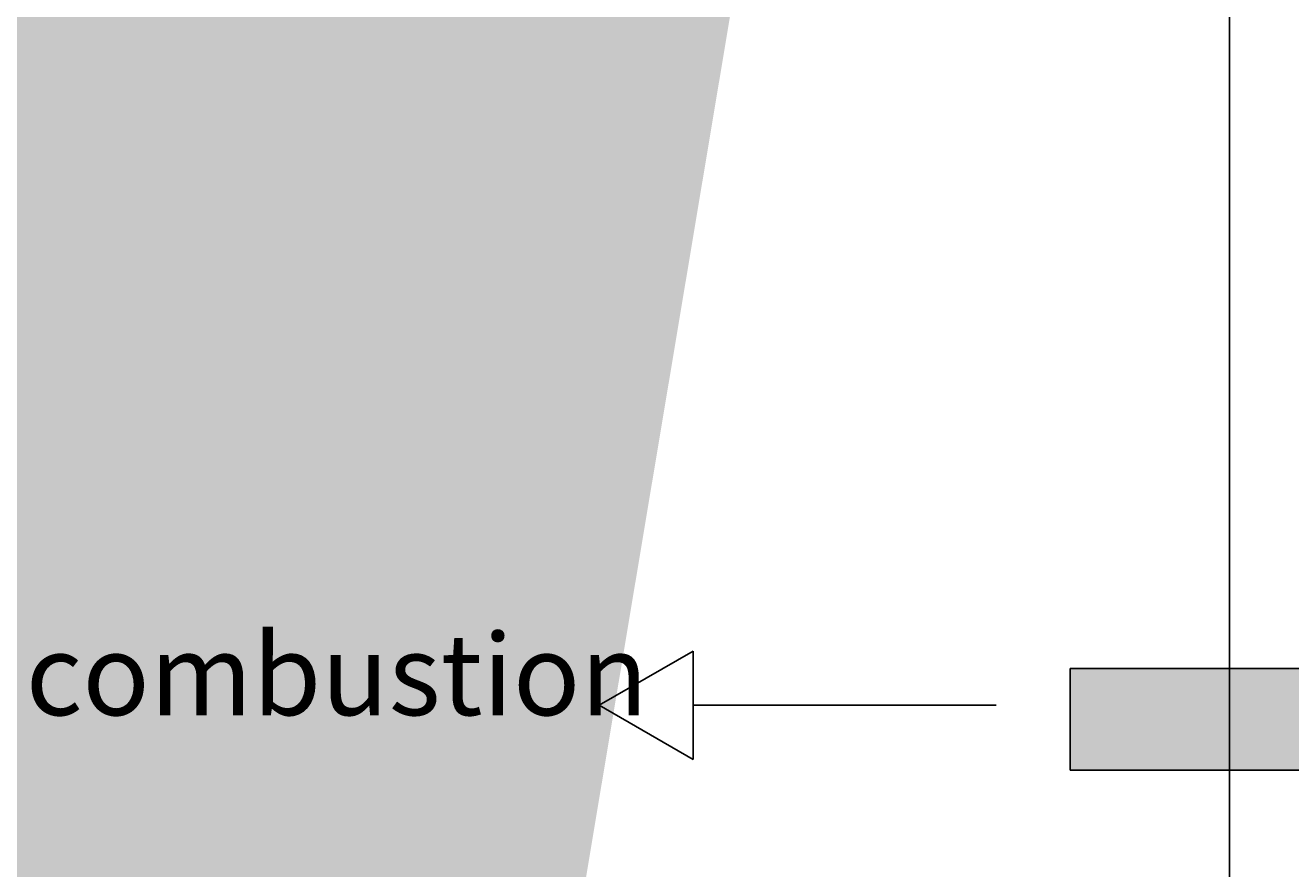
# Model space of a CAD drawing. Units: millimetres. Extents: x -22994 to 29398, y -19990 to 20176.
# Tile 25 of 135: x 37 to 99, y 138 to 180. Entities that reach past the tile are written whole.
import ezdxf

# ---------------------------------------------------------------- set-up
doc = ezdxf.new("R2010")
doc.units = ezdxf.units.MM
doc.header["$MEASUREMENT"] = 0
for name, color, linetype, lineweight in [('M-ANNO-SYMB', 7, 'Continuous', 25), ('M-ANNO-TEXT', 7, 'Continuous', 25), ('M-DIMS', 2, 'Continuous', 18), ('M-EQPM', 7, 'Continuous', 25), ('M-EQPM-PATT', 7, 'Continuous', 18)]:
    doc.layers.add(name, color=color, linetype=linetype, lineweight=lineweight)
doc.styles.get("Standard").update_dxf_attribs({"font": 'arial.ttf'})
doc.dimstyles.get("Standard").update_dxf_attribs({"dimtxt": 0.18, "dimasz": 10000, "dimexe": 0.18, "dimexo": 0.0625, "dimgap": 0.09, "dimtad": 0, "dimtih": 1, "dimtoh": 1, "dimdec": 0, "dimzin": 0, "dimdsep": 46, "dimtxsty": 'Standard', "dimcen": 0.09, "dimadec": 0, "dimazin": 0, "dimtfac": 1, "dimtdec": 0, "dimtofl": 0, "dimtmove": 0, "dimatfit": 3, "dimfxl": 1, "dimtolj": 1, "dimtzin": 0, "dimlwd": 30, "dimarcsym": 0})

# ---------------------------------------------------------------- blocks, each defined once
blk = doc.blocks.new('ARROW-FLOW')
for p, q in [((4.609, 5.322), (0, 2.661)), ((4.609, 5.322), (4.609, 0)), ((4.609, 0), (0, 2.661))]:
    blk.add_line(p, q)
blk = doc.blocks.new('*D2')
at = {"layer": 'Defpoints', "color": 0, "transparency": 16777216}
for p in [(6.677, 10.271), (290.852, 10.271), (290.852, -5.079)]:
    blk.add_point(p, dxfattribs=at)
at = {"layer": 'M-DIMS', "color": 0, "lineweight": -2, "transparency": 16777216}
for p, q in [((6.677, 10.209), (6.677, -5.259)), ((290.852, 10.209), (290.852, -5.259))]:
    blk.add_line(p, q, dxfattribs=at)
at = {"layer": 'M-DIMS', "color": 0, "lineweight": 30, "transparency": 16777216}
for p, q in [((-9993.323, -5.079), (-19993.323, -5.079)), ((10290.852, -5.079), (20290.852, -5.079))]:
    blk.add_line(p, q, dxfattribs=at)
at = {"layer": 'M-DIMS', "color": 0, "transparency": 16777216}
for points in [[(-9993.323, 1661.588), (-9993.323, -1671.745), (6.677, -5.079)], [(10290.852, 1661.588), (10290.852, -1671.745), (290.852, -5.079)]]:
    blk.add_solid(points, dxfattribs=at)
at = {"layer": 'M-DIMS', "color": 0, "transparency": 16777216, "insert": (148.765, -5.079), "char_height": 0.18, "attachment_point": 5}
blk.add_mtext('\\A1;284.2', dxfattribs=at)
blk = doc.blocks.new('*D3')
at = {"layer": 'Defpoints', "color": 0, "transparency": 16777216}
for p in [(110.265, 204.165), (110.265, 176.366), (95.833, 127.967)]:
    blk.add_point(p, dxfattribs=at)
at = {"layer": 'M-DIMS', "color": 0, "lineweight": 30, "transparency": 16777216}
for p, q in [((-9904.167, 204.165), (-19904.167, 204.165)), ((10110.265, 204.165), (20110.265, 204.165))]:
    blk.add_line(p, q, dxfattribs=at)
at = {"layer": 'M-DIMS', "color": 0, "lineweight": -2, "transparency": 16777216}
for p, q in [((95.833, 128.03), (95.833, 204.345)), ((110.265, 176.429), (110.265, 204.345))]:
    blk.add_line(p, q, dxfattribs=at)
at = {"layer": 'M-DIMS', "color": 0, "transparency": 16777216}
for points in [[(-9904.167, 1870.832), (-9904.167, -1462.501), (95.833, 204.165)], [(10110.265, 1870.832), (10110.265, -1462.501), (110.265, 204.165)]]:
    blk.add_solid(points, dxfattribs=at)
at = {"layer": 'M-DIMS', "color": 0, "transparency": 16777216, "insert": (103.049, 204.165), "char_height": 0.18, "attachment_point": 5}
blk.add_mtext('\\A1;14.432', dxfattribs=at)
blk = doc.blocks.new('*D4')
at = {"layer": 'Defpoints', "color": 0, "transparency": 16777216}
for p in [(116.265, 204.165), (110.265, 176.366), (116.265, 176.366)]:
    blk.add_point(p, dxfattribs=at)
at = {"layer": 'M-DIMS', "color": 0, "lineweight": 30, "transparency": 16777216}
for p, q in [((-9889.735, 204.165), (-19889.735, 204.165)), ((10116.265, 204.165), (20116.265, 204.165))]:
    blk.add_line(p, q, dxfattribs=at)
at = {"layer": 'M-DIMS', "color": 0, "lineweight": -2, "transparency": 16777216}
for p, q in [((110.265, 176.429), (110.265, 204.345)), ((116.265, 176.429), (116.265, 204.345))]:
    blk.add_line(p, q, dxfattribs=at)
at = {"layer": 'M-DIMS', "color": 0, "transparency": 16777216}
for points in [[(-9889.735, 1870.832), (-9889.735, -1462.501), (110.265, 204.165)], [(10116.265, 1870.832), (10116.265, -1462.501), (116.265, 204.165)]]:
    blk.add_solid(points, dxfattribs=at)
at = {"layer": 'M-DIMS', "color": 0, "transparency": 16777216, "insert": (113.265, 204.165), "char_height": 0.18, "attachment_point": 5}
blk.add_mtext('\\A1;6', dxfattribs=at)
blk = doc.blocks.new('*D5')
at = {"layer": 'Defpoints', "color": 0, "transparency": 16777216}
for p in [(181.265, 204.165), (116.265, 176.366), (181.265, 176.366)]:
    blk.add_point(p, dxfattribs=at)
at = {"layer": 'M-DIMS', "color": 0, "lineweight": 30, "transparency": 16777216}
for p, q in [((-9883.735, 204.165), (-19883.735, 204.165)), ((10181.265, 204.165), (20181.265, 204.165))]:
    blk.add_line(p, q, dxfattribs=at)
at = {"layer": 'M-DIMS', "color": 0, "lineweight": -2, "transparency": 16777216}
for p, q in [((116.265, 176.429), (116.265, 204.345)), ((181.265, 176.429), (181.265, 204.345))]:
    blk.add_line(p, q, dxfattribs=at)
at = {"layer": 'M-DIMS', "color": 0, "transparency": 16777216}
for points in [[(-9883.735, 1870.832), (-9883.735, -1462.501), (116.265, 204.165)], [(10181.265, 1870.832), (10181.265, -1462.501), (181.265, 204.165)]]:
    blk.add_solid(points, dxfattribs=at)
at = {"layer": 'M-DIMS', "color": 0, "transparency": 16777216, "insert": (148.765, 204.165), "char_height": 0.18, "attachment_point": 5}
blk.add_mtext('\\A1;65', dxfattribs=at)
blk = doc.blocks.new('*D6')
at = {"layer": 'Defpoints', "color": 0, "transparency": 16777216}
for p in [(187.265, 204.165), (181.265, 176.366), (187.265, 176.366)]:
    blk.add_point(p, dxfattribs=at)
at = {"layer": 'M-DIMS', "color": 0, "lineweight": 30, "transparency": 16777216}
for p, q in [((-9818.735, 204.165), (-19818.735, 204.165)), ((10187.265, 204.165), (20187.265, 204.165))]:
    blk.add_line(p, q, dxfattribs=at)
at = {"layer": 'M-DIMS', "color": 0, "lineweight": -2, "transparency": 16777216}
for p, q in [((181.265, 176.429), (181.265, 204.345)), ((187.265, 176.429), (187.265, 204.345))]:
    blk.add_line(p, q, dxfattribs=at)
at = {"layer": 'M-DIMS', "color": 0, "transparency": 16777216}
for points in [[(-9818.735, 1870.832), (-9818.735, -1462.501), (181.265, 204.165)], [(10187.265, 1870.832), (10187.265, -1462.501), (187.265, 204.165)]]:
    blk.add_solid(points, dxfattribs=at)
at = {"layer": 'M-DIMS', "color": 0, "transparency": 16777216, "insert": (184.265, 204.165), "char_height": 0.18, "attachment_point": 5}
blk.add_mtext('\\A1;6', dxfattribs=at)
blk = doc.blocks.new('*D7')
at = {"layer": 'Defpoints', "color": 0, "transparency": 16777216}
for p in [(201.697, 204.165), (187.265, 176.366), (201.697, 127.967)]:
    blk.add_point(p, dxfattribs=at)
at = {"layer": 'M-DIMS', "color": 0, "lineweight": 30, "transparency": 16777216}
for p, q in [((-9812.735, 204.165), (-19812.735, 204.165)), ((10201.697, 204.165), (20201.697, 204.165))]:
    blk.add_line(p, q, dxfattribs=at)
at = {"layer": 'M-DIMS', "color": 0, "lineweight": -2, "transparency": 16777216}
for p, q in [((187.265, 176.429), (187.265, 204.345)), ((201.697, 128.03), (201.697, 204.345))]:
    blk.add_line(p, q, dxfattribs=at)
at = {"layer": 'M-DIMS', "color": 0, "transparency": 16777216}
for points in [[(-9812.735, 1870.832), (-9812.735, -1462.501), (187.265, 204.165)], [(10201.697, 1870.832), (10201.697, -1462.501), (201.697, 204.165)]]:
    blk.add_solid(points, dxfattribs=at)
at = {"layer": 'M-DIMS', "color": 0, "transparency": 16777216, "insert": (194.481, 204.165), "char_height": 0.18, "attachment_point": 5}
blk.add_mtext('\\A1;14.432', dxfattribs=at)
blk = doc.blocks.new('*D8')
at = {"layer": 'Defpoints', "color": 0, "transparency": 16777216}
for p in [(227.648, 204.165), (227.648, 146.73), (201.697, 127.967)]:
    blk.add_point(p, dxfattribs=at)
at = {"layer": 'M-DIMS', "color": 0, "lineweight": 30, "transparency": 16777216}
for p, q in [((-9798.303, 204.165), (-19798.303, 204.165)), ((10227.648, 204.165), (20227.648, 204.165))]:
    blk.add_line(p, q, dxfattribs=at)
at = {"layer": 'M-DIMS', "color": 0, "lineweight": -2, "transparency": 16777216}
for p, q in [((201.697, 128.03), (201.697, 204.345)), ((227.648, 146.792), (227.648, 204.345))]:
    blk.add_line(p, q, dxfattribs=at)
at = {"layer": 'M-DIMS', "color": 0, "transparency": 16777216}
for points in [[(-9798.303, 1870.832), (-9798.303, -1462.501), (201.697, 204.165)], [(10227.648, 1870.832), (10227.648, -1462.501), (227.648, 204.165)]]:
    blk.add_solid(points, dxfattribs=at)
at = {"layer": 'M-DIMS', "color": 0, "transparency": 16777216, "insert": (214.673, 204.165), "char_height": 0.18, "attachment_point": 5}
blk.add_mtext('\\A1;25.95', dxfattribs=at)
blk = doc.blocks.new('*D9')
at = {"layer": 'Defpoints', "color": 0, "transparency": 16777216}
for p in [(187.265, 176.366), (306.202, 176.366), (290.852, 10.271)]:
    blk.add_point(p, dxfattribs=at)
at = {"layer": 'M-DIMS', "color": 0, "lineweight": 30, "transparency": 16777216}
for p, q in [((306.202, 10176.366), (306.202, 20176.366)), ((306.202, -9989.729), (306.202, -19989.729))]:
    blk.add_line(p, q, dxfattribs=at)
at = {"layer": 'M-DIMS', "color": 0, "lineweight": -2, "transparency": 16777216}
for p, q in [((187.327, 176.366), (306.382, 176.366)), ((290.915, 10.271), (306.382, 10.271))]:
    blk.add_line(p, q, dxfattribs=at)
at = {"layer": 'M-DIMS', "color": 0, "transparency": 16777216}
for points in [[(-1360.465, 10176.366), (1972.869, 10176.366), (306.202, 176.366)], [(-1360.465, -9989.729), (1972.869, -9989.729), (306.202, 10.271)]]:
    blk.add_solid(points, dxfattribs=at)
at = {"layer": 'M-DIMS', "color": 0, "transparency": 16777216, "insert": (306.202, 93.319), "char_height": 0.18, "attachment_point": 5}
blk.add_mtext('\\A1;166.1', dxfattribs=at)
blk = doc.blocks.new('*D10')
at = {"layer": 'Defpoints', "color": 0, "transparency": 16777216}
for p in [(125.65, 136.071), (133.346, 136.071), (133.346, -5.079)]:
    blk.add_point(p, dxfattribs=at)
at = {"layer": 'M-DIMS', "color": 0, "lineweight": -2, "transparency": 16777216}
for p, q in [((125.65, 136.009), (125.65, -5.259)), ((133.346, 136.009), (133.346, -5.259))]:
    blk.add_line(p, q, dxfattribs=at)
at = {"layer": 'M-DIMS', "color": 0, "lineweight": 30, "transparency": 16777216}
for p, q in [((-9874.35, -5.079), (-19874.35, -5.079)), ((10133.346, -5.079), (20133.346, -5.079))]:
    blk.add_line(p, q, dxfattribs=at)
at = {"layer": 'M-DIMS', "color": 0, "transparency": 16777216}
for points in [[(-9874.35, 1661.588), (-9874.35, -1671.745), (125.65, -5.079)], [(10133.346, 1661.588), (10133.346, -1671.745), (133.346, -5.079)]]:
    blk.add_solid(points, dxfattribs=at)
at = {"layer": 'M-DIMS', "color": 0, "transparency": 16777216, "insert": (129.498, -5.079), "char_height": 0.18, "attachment_point": 5}
blk.add_mtext('\\A1;7.696', dxfattribs=at)
blk = doc.blocks.new('*D11')
at = {"layer": 'Defpoints', "color": 0, "transparency": 16777216}
for p in [(133.346, 136.071), (135.65, 136.071), (135.65, -5.079)]:
    blk.add_point(p, dxfattribs=at)
at = {"layer": 'M-DIMS', "color": 0, "lineweight": -2, "transparency": 16777216}
for p, q in [((133.346, 136.009), (133.346, -5.259)), ((135.65, 136.009), (135.65, -5.259))]:
    blk.add_line(p, q, dxfattribs=at)
at = {"layer": 'M-DIMS', "color": 0, "lineweight": 30, "transparency": 16777216}
for p, q in [((-9866.654, -5.079), (-19866.654, -5.079)), ((10135.65, -5.079), (20135.65, -5.079))]:
    blk.add_line(p, q, dxfattribs=at)
at = {"layer": 'M-DIMS', "color": 0, "transparency": 16777216}
for points in [[(-9866.654, 1661.588), (-9866.654, -1671.745), (133.346, -5.079)], [(10135.65, 1661.588), (10135.65, -1671.745), (135.65, -5.079)]]:
    blk.add_solid(points, dxfattribs=at)
at = {"layer": 'M-DIMS', "color": 0, "transparency": 16777216, "insert": (134.498, -5.079), "char_height": 0.18, "attachment_point": 5}
blk.add_mtext('\\A1;2.304', dxfattribs=at)
blk = doc.blocks.new('*D12')
at = {"layer": 'Defpoints', "color": 0, "transparency": 16777216}
for p in [(135.65, 136.071), (145.65, 136.071), (145.65, -5.079)]:
    blk.add_point(p, dxfattribs=at)
at = {"layer": 'M-DIMS', "color": 0, "lineweight": -2, "transparency": 16777216}
for p, q in [((135.65, 136.009), (135.65, -5.259)), ((145.65, 136.009), (145.65, -5.259))]:
    blk.add_line(p, q, dxfattribs=at)
at = {"layer": 'M-DIMS', "color": 0, "lineweight": 30, "transparency": 16777216}
for p, q in [((-9864.35, -5.079), (-19864.35, -5.079)), ((10145.65, -5.079), (20145.65, -5.079))]:
    blk.add_line(p, q, dxfattribs=at)
at = {"layer": 'M-DIMS', "color": 0, "transparency": 16777216}
for points in [[(-9864.35, 1661.588), (-9864.35, -1671.745), (135.65, -5.079)], [(10145.65, 1661.588), (10145.65, -1671.745), (145.65, -5.079)]]:
    blk.add_solid(points, dxfattribs=at)
at = {"layer": 'M-DIMS', "color": 0, "transparency": 16777216, "insert": (140.65, -5.079), "char_height": 0.18, "attachment_point": 5}
blk.add_mtext('\\A1;10', dxfattribs=at)
blk = doc.blocks.new('*D13')
at = {"layer": 'Defpoints', "color": 0, "transparency": 16777216}
for p in [(145.65, 136.071), (155.65, 136.071), (155.65, -5.079)]:
    blk.add_point(p, dxfattribs=at)
at = {"layer": 'M-DIMS', "color": 0, "lineweight": -2, "transparency": 16777216}
for p, q in [((145.65, 136.009), (145.65, -5.259)), ((155.65, 136.009), (155.65, -5.259))]:
    blk.add_line(p, q, dxfattribs=at)
at = {"layer": 'M-DIMS', "color": 0, "lineweight": 30, "transparency": 16777216}
for p, q in [((-9854.35, -5.079), (-19854.35, -5.079)), ((10155.65, -5.079), (20155.65, -5.079))]:
    blk.add_line(p, q, dxfattribs=at)
at = {"layer": 'M-DIMS', "color": 0, "transparency": 16777216}
for points in [[(-9854.35, 1661.588), (-9854.35, -1671.745), (145.65, -5.079)], [(10155.65, 1661.588), (10155.65, -1671.745), (155.65, -5.079)]]:
    blk.add_solid(points, dxfattribs=at)
at = {"layer": 'M-DIMS', "color": 0, "transparency": 16777216, "insert": (150.65, -5.079), "char_height": 0.18, "attachment_point": 5}
blk.add_mtext('\\A1;10', dxfattribs=at)
blk = doc.blocks.new('*D14')
at = {"layer": 'Defpoints', "color": 0, "transparency": 16777216}
for p in [(155.65, 136.071), (165.65, 136.071), (165.65, -5.079)]:
    blk.add_point(p, dxfattribs=at)
at = {"layer": 'M-DIMS', "color": 0, "lineweight": -2, "transparency": 16777216}
for p, q in [((155.65, 136.009), (155.65, -5.259)), ((165.65, 136.009), (165.65, -5.259))]:
    blk.add_line(p, q, dxfattribs=at)
at = {"layer": 'M-DIMS', "color": 0, "lineweight": 30, "transparency": 16777216}
for p, q in [((-9844.35, -5.079), (-19844.35, -5.079)), ((10165.65, -5.079), (20165.65, -5.079))]:
    blk.add_line(p, q, dxfattribs=at)
at = {"layer": 'M-DIMS', "color": 0, "transparency": 16777216}
for points in [[(-9844.35, 1661.588), (-9844.35, -1671.745), (155.65, -5.079)], [(10165.65, 1661.588), (10165.65, -1671.745), (165.65, -5.079)]]:
    blk.add_solid(points, dxfattribs=at)
at = {"layer": 'M-DIMS', "color": 0, "transparency": 16777216, "insert": (160.65, -5.079), "char_height": 0.18, "attachment_point": 5}
blk.add_mtext('\\A1;10', dxfattribs=at)
blk = doc.blocks.new('*D15')
at = {"layer": 'Defpoints', "color": 0, "transparency": 16777216}
for p in [(173.346, 154.788), (173.346, 136.071), (306.202, 136.071)]:
    blk.add_point(p, dxfattribs=at)
at = {"layer": 'M-DIMS', "color": 0, "lineweight": 30, "transparency": 16777216}
for p, q in [((306.202, 10154.788), (306.202, 20154.788)), ((306.202, -9863.929), (306.202, -19863.929))]:
    blk.add_line(p, q, dxfattribs=at)
at = {"layer": 'M-DIMS', "color": 0, "lineweight": -2, "transparency": 16777216}
for p, q in [((173.408, 154.788), (306.382, 154.788)), ((173.408, 136.071), (306.382, 136.071))]:
    blk.add_line(p, q, dxfattribs=at)
at = {"layer": 'M-DIMS', "color": 0, "transparency": 16777216}
for points in [[(-1360.465, 10154.788), (1972.869, 10154.788), (306.202, 154.788)], [(-1360.465, -9863.929), (1972.869, -9863.929), (306.202, 136.071)]]:
    blk.add_solid(points, dxfattribs=at)
at = {"layer": 'M-DIMS', "color": 0, "transparency": 16777216, "insert": (306.202, 145.43), "char_height": 0.18, "attachment_point": 5}
blk.add_mtext('\\A1;18.717', dxfattribs=at)
blk = doc.blocks.new('*D16')
at = {"layer": 'Defpoints', "color": 0, "transparency": 16777216}
for p in [(120.17, 204.165), (110.466, 48.035), (120.17, 48.035)]:
    blk.add_point(p, dxfattribs=at)
at = {"layer": 'M-DIMS', "color": 0, "lineweight": 30, "transparency": 16777216}
for p, q in [((-9889.534, 204.165), (-19889.534, 204.165)), ((10120.17, 204.165), (20120.17, 204.165))]:
    blk.add_line(p, q, dxfattribs=at)
at = {"layer": 'M-DIMS', "color": 0, "lineweight": -2, "transparency": 16777216}
for p, q in [((110.466, 48.097), (110.466, 204.345)), ((120.17, 48.097), (120.17, 204.345))]:
    blk.add_line(p, q, dxfattribs=at)
at = {"layer": 'M-DIMS', "color": 0, "transparency": 16777216}
for points in [[(-9889.534, 1870.832), (-9889.534, -1462.501), (110.466, 204.165)], [(10120.17, 1870.832), (10120.17, -1462.501), (120.17, 204.165)]]:
    blk.add_solid(points, dxfattribs=at)
at = {"layer": 'M-DIMS', "color": 0, "transparency": 16777216, "insert": (115.318, 204.165), "char_height": 0.18, "attachment_point": 5}
blk.add_mtext('\\A1;9.704', dxfattribs=at)
blk = doc.blocks.new('*D17')
at = {"layer": 'Defpoints', "color": 0, "transparency": 16777216}
for p in [(126.17, 204.165), (120.17, 48.035), (126.17, 48.035)]:
    blk.add_point(p, dxfattribs=at)
at = {"layer": 'M-DIMS', "color": 0, "lineweight": 30, "transparency": 16777216}
for p, q in [((-9879.83, 204.165), (-19879.83, 204.165)), ((10126.17, 204.165), (20126.17, 204.165))]:
    blk.add_line(p, q, dxfattribs=at)
at = {"layer": 'M-DIMS', "color": 0, "lineweight": -2, "transparency": 16777216}
for p, q in [((120.17, 48.097), (120.17, 204.345)), ((126.17, 48.097), (126.17, 204.345))]:
    blk.add_line(p, q, dxfattribs=at)
at = {"layer": 'M-DIMS', "color": 0, "transparency": 16777216}
for points in [[(-9879.83, 1870.832), (-9879.83, -1462.501), (120.17, 204.165)], [(10126.17, 1870.832), (10126.17, -1462.501), (126.17, 204.165)]]:
    blk.add_solid(points, dxfattribs=at)
at = {"layer": 'M-DIMS', "color": 0, "transparency": 16777216, "insert": (123.17, 204.165), "char_height": 0.18, "attachment_point": 5}
blk.add_mtext('\\A1;6', dxfattribs=at)
blk = doc.blocks.new('*D18')
at = {"layer": 'Defpoints', "color": 0, "transparency": 16777216}
for p in [(132.17, 204.165), (126.17, 48.035), (132.17, 48.035)]:
    blk.add_point(p, dxfattribs=at)
at = {"layer": 'M-DIMS', "color": 0, "lineweight": 30, "transparency": 16777216}
for p, q in [((-9873.83, 204.165), (-19873.83, 204.165)), ((10132.17, 204.165), (20132.17, 204.165))]:
    blk.add_line(p, q, dxfattribs=at)
at = {"layer": 'M-DIMS', "color": 0, "lineweight": -2, "transparency": 16777216}
for p, q in [((126.17, 48.097), (126.17, 204.345)), ((132.17, 48.097), (132.17, 204.345))]:
    blk.add_line(p, q, dxfattribs=at)
at = {"layer": 'M-DIMS', "color": 0, "transparency": 16777216}
for points in [[(-9873.83, 1870.832), (-9873.83, -1462.501), (126.17, 204.165)], [(10132.17, 1870.832), (10132.17, -1462.501), (132.17, 204.165)]]:
    blk.add_solid(points, dxfattribs=at)
at = {"layer": 'M-DIMS', "color": 0, "transparency": 16777216, "insert": (129.17, 204.165), "char_height": 0.18, "attachment_point": 5}
blk.add_mtext('\\A1;6', dxfattribs=at)
blk = doc.blocks.new('*D19')
at = {"layer": 'Defpoints', "color": 0, "transparency": 16777216}
for p in [(138.17, 204.165), (132.17, 48.035), (138.17, 48.035)]:
    blk.add_point(p, dxfattribs=at)
at = {"layer": 'M-DIMS', "color": 0, "lineweight": 30, "transparency": 16777216}
for p, q in [((-9867.83, 204.165), (-19867.83, 204.165)), ((10138.17, 204.165), (20138.17, 204.165))]:
    blk.add_line(p, q, dxfattribs=at)
at = {"layer": 'M-DIMS', "color": 0, "lineweight": -2, "transparency": 16777216}
for p, q in [((132.17, 48.097), (132.17, 204.345)), ((138.17, 48.097), (138.17, 204.345))]:
    blk.add_line(p, q, dxfattribs=at)
at = {"layer": 'M-DIMS', "color": 0, "transparency": 16777216}
for points in [[(-9867.83, 1870.832), (-9867.83, -1462.501), (132.17, 204.165)], [(10138.17, 1870.832), (10138.17, -1462.501), (138.17, 204.165)]]:
    blk.add_solid(points, dxfattribs=at)
at = {"layer": 'M-DIMS', "color": 0, "transparency": 16777216, "insert": (135.17, 204.165), "char_height": 0.18, "attachment_point": 5}
blk.add_mtext('\\A1;6', dxfattribs=at)
blk = doc.blocks.new('*D20')
at = {"layer": 'Defpoints', "color": 0, "transparency": 16777216}
for p in [(144.17, 204.165), (138.17, 48.035), (144.17, 48.035)]:
    blk.add_point(p, dxfattribs=at)
at = {"layer": 'M-DIMS', "color": 0, "lineweight": 30, "transparency": 16777216}
for p, q in [((-9861.83, 204.165), (-19861.83, 204.165)), ((10144.17, 204.165), (20144.17, 204.165))]:
    blk.add_line(p, q, dxfattribs=at)
at = {"layer": 'M-DIMS', "color": 0, "lineweight": -2, "transparency": 16777216}
for p, q in [((138.17, 48.097), (138.17, 204.345)), ((144.17, 48.097), (144.17, 204.345))]:
    blk.add_line(p, q, dxfattribs=at)
at = {"layer": 'M-DIMS', "color": 0, "transparency": 16777216}
for points in [[(-9861.83, 1870.832), (-9861.83, -1462.501), (138.17, 204.165)], [(10144.17, 1870.832), (10144.17, -1462.501), (144.17, 204.165)]]:
    blk.add_solid(points, dxfattribs=at)
at = {"layer": 'M-DIMS', "color": 0, "transparency": 16777216, "insert": (141.17, 204.165), "char_height": 0.18, "attachment_point": 5}
blk.add_mtext('\\A1;6', dxfattribs=at)
blk = doc.blocks.new('*D21')
at = {"layer": 'Defpoints', "color": 0, "transparency": 16777216}
for p in [(149.116, 204.165), (144.17, 48.035), (149.116, 48.035)]:
    blk.add_point(p, dxfattribs=at)
at = {"layer": 'M-DIMS', "color": 0, "lineweight": 30, "transparency": 16777216}
for p, q in [((-9855.83, 204.165), (-19855.83, 204.165)), ((10149.116, 204.165), (20149.116, 204.165))]:
    blk.add_line(p, q, dxfattribs=at)
at = {"layer": 'M-DIMS', "color": 0, "lineweight": -2, "transparency": 16777216}
for p, q in [((144.17, 48.097), (144.17, 204.345)), ((149.116, 48.097), (149.116, 204.345))]:
    blk.add_line(p, q, dxfattribs=at)
at = {"layer": 'M-DIMS', "color": 0, "transparency": 16777216}
for points in [[(-9855.83, 1870.832), (-9855.83, -1462.501), (144.17, 204.165)], [(10149.116, 1870.832), (10149.116, -1462.501), (149.116, 204.165)]]:
    blk.add_solid(points, dxfattribs=at)
at = {"layer": 'M-DIMS', "color": 0, "transparency": 16777216, "insert": (146.643, 204.165), "char_height": 0.18, "attachment_point": 5}
blk.add_mtext('\\A1;4.945', dxfattribs=at)
blk = doc.blocks.new('*D22')
at = {"layer": 'Defpoints', "color": 0, "transparency": 16777216}
for p in [(149.116, 30.99), (155.116, 30.99), (155.116, -5.079)]:
    blk.add_point(p, dxfattribs=at)
at = {"layer": 'M-DIMS', "color": 0, "lineweight": -2, "transparency": 16777216}
for p, q in [((149.116, 30.927), (149.116, -5.259)), ((155.116, 30.927), (155.116, -5.259))]:
    blk.add_line(p, q, dxfattribs=at)
at = {"layer": 'M-DIMS', "color": 0, "lineweight": 30, "transparency": 16777216}
for p, q in [((-9850.884, -5.079), (-19850.884, -5.079)), ((10155.116, -5.079), (20155.116, -5.079))]:
    blk.add_line(p, q, dxfattribs=at)
at = {"layer": 'M-DIMS', "color": 0, "transparency": 16777216}
for points in [[(-9850.884, 1661.588), (-9850.884, -1671.745), (149.116, -5.079)], [(10155.116, 1661.588), (10155.116, -1671.745), (155.116, -5.079)]]:
    blk.add_solid(points, dxfattribs=at)
at = {"layer": 'M-DIMS', "color": 0, "transparency": 16777216, "insert": (152.116, -5.079), "char_height": 0.18, "attachment_point": 5}
blk.add_mtext('\\A1;6', dxfattribs=at)
blk = doc.blocks.new('*D23')
at = {"layer": 'Defpoints', "color": 0, "transparency": 16777216}
for p in [(155.116, 30.99), (161.116, 30.99), (161.116, -5.079)]:
    blk.add_point(p, dxfattribs=at)
at = {"layer": 'M-DIMS', "color": 0, "lineweight": -2, "transparency": 16777216}
for p, q in [((155.116, 30.927), (155.116, -5.259)), ((161.116, 30.927), (161.116, -5.259))]:
    blk.add_line(p, q, dxfattribs=at)
at = {"layer": 'M-DIMS', "color": 0, "lineweight": 30, "transparency": 16777216}
for p, q in [((-9844.884, -5.079), (-19844.884, -5.079)), ((10161.116, -5.079), (20161.116, -5.079))]:
    blk.add_line(p, q, dxfattribs=at)
at = {"layer": 'M-DIMS', "color": 0, "transparency": 16777216}
for points in [[(-9844.884, 1661.588), (-9844.884, -1671.745), (155.116, -5.079)], [(10161.116, 1661.588), (10161.116, -1671.745), (161.116, -5.079)]]:
    blk.add_solid(points, dxfattribs=at)
at = {"layer": 'M-DIMS', "color": 0, "transparency": 16777216, "insert": (158.116, -5.079), "char_height": 0.18, "attachment_point": 5}
blk.add_mtext('\\A1;6', dxfattribs=at)
blk = doc.blocks.new('*D24')
at = {"layer": 'Defpoints', "color": 0, "transparency": 16777216}
for p in [(161.116, 30.99), (166.439, 30.99), (166.439, -5.079)]:
    blk.add_point(p, dxfattribs=at)
at = {"layer": 'M-DIMS', "color": 0, "lineweight": -2, "transparency": 16777216}
for p, q in [((161.116, 30.927), (161.116, -5.259)), ((166.439, 30.927), (166.439, -5.259))]:
    blk.add_line(p, q, dxfattribs=at)
at = {"layer": 'M-DIMS', "color": 0, "lineweight": 30, "transparency": 16777216}
for p, q in [((-9838.884, -5.079), (-19838.884, -5.079)), ((10166.439, -5.079), (20166.439, -5.079))]:
    blk.add_line(p, q, dxfattribs=at)
at = {"layer": 'M-DIMS', "color": 0, "transparency": 16777216}
for points in [[(-9838.884, 1661.588), (-9838.884, -1671.745), (161.116, -5.079)], [(10166.439, 1661.588), (10166.439, -1671.745), (166.439, -5.079)]]:
    blk.add_solid(points, dxfattribs=at)
at = {"layer": 'M-DIMS', "color": 0, "transparency": 16777216, "insert": (163.777, -5.079), "char_height": 0.18, "attachment_point": 5}
blk.add_mtext('\\A1;5.323', dxfattribs=at)
blk = doc.blocks.new('*D25')
at = {"layer": 'Defpoints', "color": 0, "transparency": 16777216}
for p in [(166.439, 30.99), (172.439, 30.99), (172.439, -5.079)]:
    blk.add_point(p, dxfattribs=at)
at = {"layer": 'M-DIMS', "color": 0, "lineweight": -2, "transparency": 16777216}
for p, q in [((166.439, 30.927), (166.439, -5.259)), ((172.439, 30.927), (172.439, -5.259))]:
    blk.add_line(p, q, dxfattribs=at)
at = {"layer": 'M-DIMS', "color": 0, "lineweight": 30, "transparency": 16777216}
for p, q in [((-9833.561, -5.079), (-19833.561, -5.079)), ((10172.439, -5.079), (20172.439, -5.079))]:
    blk.add_line(p, q, dxfattribs=at)
at = {"layer": 'M-DIMS', "color": 0, "transparency": 16777216}
for points in [[(-9833.561, 1661.588), (-9833.561, -1671.745), (166.439, -5.079)], [(10172.439, 1661.588), (10172.439, -1671.745), (172.439, -5.079)]]:
    blk.add_solid(points, dxfattribs=at)
at = {"layer": 'M-DIMS', "color": 0, "transparency": 16777216, "insert": (169.439, -5.079), "char_height": 0.18, "attachment_point": 5}
blk.add_mtext('\\A1;6', dxfattribs=at)
blk = doc.blocks.new('*D26')
at = {"layer": 'Defpoints', "color": 0, "transparency": 16777216}
for p in [(172.439, 30.99), (178.439, 30.99), (178.439, -5.079)]:
    blk.add_point(p, dxfattribs=at)
at = {"layer": 'M-DIMS', "color": 0, "lineweight": -2, "transparency": 16777216}
for p, q in [((172.439, 30.927), (172.439, -5.259)), ((178.439, 30.927), (178.439, -5.259))]:
    blk.add_line(p, q, dxfattribs=at)
at = {"layer": 'M-DIMS', "color": 0, "lineweight": 30, "transparency": 16777216}
for p, q in [((-9827.561, -5.079), (-19827.561, -5.079)), ((10178.439, -5.079), (20178.439, -5.079))]:
    blk.add_line(p, q, dxfattribs=at)
at = {"layer": 'M-DIMS', "color": 0, "transparency": 16777216}
for points in [[(-9827.561, 1661.588), (-9827.561, -1671.745), (172.439, -5.079)], [(10178.439, 1661.588), (10178.439, -1671.745), (178.439, -5.079)]]:
    blk.add_solid(points, dxfattribs=at)
at = {"layer": 'M-DIMS', "color": 0, "transparency": 16777216, "insert": (175.439, -5.079), "char_height": 0.18, "attachment_point": 5}
blk.add_mtext('\\A1;6', dxfattribs=at)
blk = doc.blocks.new('*D27')
at = {"layer": 'Defpoints', "color": 0, "transparency": 16777216}
for p in [(178.439, 30.99), (188.117, 30.99), (188.117, -5.079)]:
    blk.add_point(p, dxfattribs=at)
at = {"layer": 'M-DIMS', "color": 0, "lineweight": -2, "transparency": 16777216}
for p, q in [((178.439, 30.927), (178.439, -5.259)), ((188.117, 30.927), (188.117, -5.259))]:
    blk.add_line(p, q, dxfattribs=at)
at = {"layer": 'M-DIMS', "color": 0, "lineweight": 30, "transparency": 16777216}
for p, q in [((-9821.561, -5.079), (-19821.561, -5.079)), ((10188.117, -5.079), (20188.117, -5.079))]:
    blk.add_line(p, q, dxfattribs=at)
at = {"layer": 'M-DIMS', "color": 0, "transparency": 16777216}
for points in [[(-9821.561, 1661.588), (-9821.561, -1671.745), (178.439, -5.079)], [(10188.117, 1661.588), (10188.117, -1671.745), (188.117, -5.079)]]:
    blk.add_solid(points, dxfattribs=at)
at = {"layer": 'M-DIMS', "color": 0, "transparency": 16777216, "insert": (183.278, -5.079), "char_height": 0.18, "attachment_point": 5}
blk.add_mtext('\\A1;9.679', dxfattribs=at)
blk = doc.blocks.new('*D28')
at = {"layer": 'Defpoints', "color": 0, "transparency": 16777216}
for p in [(188.117, 48.035), (306.202, 48.035), (188.117, 30.99)]:
    blk.add_point(p, dxfattribs=at)
at = {"layer": 'M-DIMS', "color": 0, "lineweight": 30, "transparency": 16777216}
for p, q in [((306.202, 10048.035), (306.202, 20048.035)), ((306.202, -9969.01), (306.202, -19969.01))]:
    blk.add_line(p, q, dxfattribs=at)
at = {"layer": 'M-DIMS', "color": 0, "lineweight": -2, "transparency": 16777216}
for p, q in [((188.18, 48.035), (306.382, 48.035)), ((188.18, 30.99), (306.382, 30.99))]:
    blk.add_line(p, q, dxfattribs=at)
at = {"layer": 'M-DIMS', "color": 0, "transparency": 16777216}
for points in [[(-1360.465, 10048.035), (1972.869, 10048.035), (306.202, 48.035)], [(-1360.465, -9969.01), (1972.869, -9969.01), (306.202, 30.99)]]:
    blk.add_solid(points, dxfattribs=at)
at = {"layer": 'M-DIMS', "color": 0, "transparency": 16777216, "insert": (306.202, 39.512), "char_height": 0.18, "attachment_point": 5}
blk.add_mtext('\\A1;17.045', dxfattribs=at)
blk = doc.blocks.new('*D29')
at = {"layer": 'Defpoints', "color": 0, "transparency": 16777216}
for p in [(36.801, 80.045), (64.03, 80.045)]:
    blk.add_point(p, dxfattribs=at)
at = {"layer": 'M-DIMS', "color": 0, "lineweight": -2, "transparency": 16777216}
for p, q in [((50.325, 80.045), (50.505, 80.045)), ((50.415, 79.955), (50.415, 80.135))]:
    blk.add_line(p, q, dxfattribs=at)
at = {"layer": 'M-DIMS', "color": 0, "lineweight": 30, "transparency": 16777216}
blk.add_line((20064.03, 80.03), (10064.03, 80.038), dxfattribs=at)
at = {"layer": 'M-DIMS', "color": 0, "transparency": 16777216}
blk.add_solid([(10064.031, 1746.704), (10064.028, -1586.629), (64.03, 80.045)], dxfattribs=at)
at = {"layer": 'M-DIMS', "color": 0, "transparency": 16777216, "insert": (20064.521, 80.03), "char_height": 0.18, "attachment_point": 5}
blk.add_mtext('\\A1;∅27.23', dxfattribs=at)
blk = doc.blocks.new('*D36')
at = {"layer": 'Defpoints', "color": 0, "transparency": 16777216}
for p in [(46.39, 31.303), (46.387, 26.593)]:
    blk.add_point(p, dxfattribs=at)
at = {"layer": 'M-DIMS', "color": 0, "lineweight": 30, "transparency": 16777216}
for p, q in [((57.15, 20031.301), (51.77, 10031.302)), ((10057.15, 20031.301), (57.15, 20031.301))]:
    blk.add_line(p, q, dxfattribs=at)
at = {"layer": 'M-DIMS', "color": 0, "lineweight": -2, "transparency": 16777216}
for p, q in [((46.299, 28.948), (46.479, 28.948)), ((46.389, 28.858), (46.389, 29.038))]:
    blk.add_line(p, q, dxfattribs=at)
at = {"layer": 'M-DIMS', "color": 0, "transparency": 16777216}
blk.add_solid([(-1614.896, 10032.199), (1718.436, 10030.405), (46.39, 31.303)], dxfattribs=at)
at = {"layer": 'M-DIMS', "color": 0, "transparency": 16777216, "insert": (10057.554, 20031.301), "char_height": 0.18, "attachment_point": 5}
blk.add_mtext('\\A1;∅4.71', dxfattribs=at)
blk = doc.blocks.new('*D37')
at = {"layer": 'Defpoints', "color": 0, "transparency": 16777216}
for p in [(54.834, 118.615), (59.494, 118.614)]:
    blk.add_point(p, dxfattribs=at)
at = {"layer": 'M-DIMS', "color": 0, "lineweight": -2, "transparency": 16777216}
for p, q in [((57.074, 118.614), (57.254, 118.614)), ((57.164, 118.524), (57.164, 118.704))]:
    blk.add_line(p, q, dxfattribs=at)
at = {"layer": 'M-DIMS', "color": 0, "lineweight": 30, "transparency": 16777216}
blk.add_line((20059.493, 116.253), (10059.494, 117.434), dxfattribs=at)
at = {"layer": 'M-DIMS', "color": 0, "transparency": 16777216}
blk.add_solid([(10059.69, 1784.1), (10059.297, -1549.233), (59.494, 118.614)], dxfattribs=at)
at = {"layer": 'M-DIMS', "color": 0, "transparency": 16777216, "insert": (20059.985, 116.253), "char_height": 0.18, "attachment_point": 5}
blk.add_mtext('\\A1;∅4.659', dxfattribs=at)

msp = doc.modelspace()

# ---------------------------------------------------------------- hatches: boundary and pattern name
at = {"layer": 'M-EQPM-PATT'}
h = msp.add_hatch(color=256, dxfattribs=at)
h.set_gradient(color1=(128, 128, 128), color2=(128, 128, 128), tint=1)
h.paths.add_polyline_path([(88.0003, 148.1301), (88.0003, 143.1301), (104.9278, 143.1301), (107.9269, 148.1301)])
h.paths.add_polyline_path([(189.6025, 148.1301), (192.6016, 143.1301), (216.9016, 143.1301, -0.0809736), (216.3148, 146.7296, -0.0309822), (216.4017, 148.1301)])
h.paths.add_polyline_path([(229.9653, 167.6546), (245.0476, 167.6546), (245.0476, 172.6546), (224.9653, 172.6546), (224.9653, 157.741, -0.1116822), (229.9653, 157.8239)])
h.paths.add_polyline_path([(36.3887, 21.6644), (36.3887, 16.6063), (56.3887, 16.6063), (56.3887, 21.6644)])

# ---------------------------------------------------------------- linework, layer by layer
at = {"layer": 'M-ANNO-SYMB'}
msp.add_line((69.4699, 146.318), (84.3614, 146.318), dxfattribs=at)
at = {"layer": 'M-EQPM'}
for p, q in [((88.0003, 148.1301), (88.0003, 143.1301)), ((107.9269, 148.1301), (88.0003, 148.1301)), ((88.0003, 143.1301), (104.9278, 143.1301))]:
    msp.add_line(p, q, dxfattribs=at)

# ---------------------------------------------------------------- block references
at = {"layer": 'M-ANNO-SYMB'}
msp.add_blockref('ARROW-FLOW', (64.861, 143.657), dxfattribs=at)

# ---------------------------------------------------------------- texts
at = {"layer": 'M-ANNO-TEXT', "insert": (11.6233, 149.8324), "char_height": 4, "attachment_point": 1}
msp.add_mtext_dynamic_manual_height_columns('Hot air to combustion chamber', width=57.451589, gutter_width=1, heights=[0], dxfattribs=at)

# ---------------------------------------------------------------- dimensions: what is measured, and where the dimension line sits
at = {"layer": 'M-DIMS'}
for base, p1, p2, override, picture, middle in [((306.202, 176.3662), (290.852, 10.2713), (187.2647, 176.3662), {"dimdec": 1, "dimlfac": 1, "dimrnd": 0, "dimzin": 0, "dimdsep": 46, "dimlunit": 2}, '*D9', (306.202, 93.3187)), ((306.202, 136.0713), (173.3459, 154.788), (173.3459, 136.0713), {"dimdec": 3, "dimlfac": 1, "dimrnd": 0, "dimzin": 0, "dimdsep": 46, "dimlunit": 2}, '*D15', (306.202, 145.4297)), ((306.202, 48.0349), (188.1175, 30.9895), (188.1175, 48.0349), {"dimdec": 3, "dimlfac": 1, "dimrnd": 0, "dimzin": 0, "dimdsep": 46, "dimlunit": 2}, '*D28', (306.202, 39.5122))]:
    dim = msp.add_linear_dim(base=base, p1=p1, p2=p2, angle=90, dimstyle='Standard', override=override, dxfattribs=at)
    dim.commit()
    dim.dimension.update_dxf_attribs({"geometry": picture, "text_midpoint": middle})
dim = msp.add_diameter_dim_2p(p1=(46.3875, 26.5934), p2=(46.39, 31.3035), dimstyle='Standard', override={"dimdec": 2, "dimlfac": 1, "dimrnd": 0, "dimzin": 0, "dimdsep": 46, "dimlunit": 2}, dxfattribs=at)
dim.commit()
dim.dimension.update_dxf_attribs({"geometry": '*D36', "text_midpoint": (10057.5542, 20031.3006), "dimtype": 163})
for base, p1, p2, override, picture, middle in [((110.2647, 204.1654), (95.8327, 127.967), (110.2647, 176.3662), {"dimdec": 3, "dimlfac": 1, "dimrnd": 0, "dimzin": 0, "dimdsep": 46, "dimlunit": 2}, '*D3', (103.0487, 204.1654)), ((116.2647, 204.1654), (110.2647, 176.3662), (116.2647, 176.3662), {"dimdec": 0, "dimlfac": 1, "dimrnd": 0, "dimzin": 0, "dimdsep": 46, "dimlunit": 2}, '*D4', (113.2647, 204.1654)), ((120.1702, 204.1654), (110.4658, 48.0349), (120.1702, 48.0349), {"dimdec": 3, "dimlfac": 1, "dimrnd": 0, "dimzin": 0, "dimdsep": 46, "dimlunit": 2}, '*D16', (115.318, 204.1654)), ((181.2647, 204.1654), (116.2647, 176.3662), (181.2647, 176.3662), {"dimdec": 0, "dimlfac": 1, "dimrnd": 0, "dimzin": 0, "dimdsep": 46, "dimlunit": 2}, '*D5', (148.7647, 204.1654)), ((126.1702, 204.1654), (120.1702, 48.0349), (126.1702, 48.0349), {"dimdec": 0, "dimlfac": 1, "dimrnd": 0, "dimzin": 0, "dimdsep": 46, "dimlunit": 2}, '*D17', (123.1702, 204.1654)), ((132.1702, 204.1654), (126.1702, 48.0349), (132.1702, 48.0349), {"dimdec": 0, "dimlfac": 1, "dimrnd": 0, "dimzin": 0, "dimdsep": 46, "dimlunit": 2}, '*D18', (129.1702, 204.1654)), ((138.1702, 204.1654), (132.1702, 48.0349), (138.1702, 48.0349), {"dimdec": 0, "dimlfac": 1, "dimrnd": 0, "dimzin": 0, "dimdsep": 46, "dimlunit": 2}, '*D19', (135.1702, 204.1654)), ((144.1702, 204.1654), (138.1702, 48.0349), (144.1702, 48.0349), {"dimdec": 0, "dimlfac": 1, "dimrnd": 0, "dimzin": 0, "dimdsep": 46, "dimlunit": 2}, '*D20', (141.1702, 204.1654)), ((149.11567, 204.16539), (144.17023, 48.03494), (149.11567, 48.03494), {"dimdec": 3, "dimlfac": 1, "dimrnd": 0, "dimzin": 0, "dimdsep": 46, "dimlunit": 2}, '*D21', (146.64295, 204.16539)), ((187.2647, 204.1654), (181.2647, 176.3662), (187.2647, 176.3662), {"dimdec": 0, "dimlfac": 1, "dimrnd": 0, "dimzin": 0, "dimdsep": 46, "dimlunit": 2}, '*D6', (184.2647, 204.1654)), ((201.6967, 204.1654), (187.2647, 176.3662), (201.6967, 127.967), {"dimdec": 3, "dimlfac": 1, "dimrnd": 0, "dimzin": 0, "dimdsep": 46, "dimlunit": 2}, '*D7', (194.4807, 204.1654)), ((227.6485, 204.1654), (201.6967, 127.967), (227.6485, 146.7296), {"dimdec": 2, "dimlfac": 1, "dimrnd": 0, "dimzin": 0, "dimdsep": 46, "dimlunit": 2}, '*D8', (214.6726, 204.1654)), ((290.852, -5.0787), (6.6773, 10.2713), (290.852, 10.2713), {"dimdec": 1, "dimlfac": 1, "dimrnd": 0, "dimzin": 0, "dimdsep": 46, "dimlunit": 2}, '*D2', (148.7647, -5.0787)), ((133.3459, -5.0787), (125.6498, 136.0713), (133.3459, 136.0713), {"dimdec": 3, "dimlfac": 1, "dimrnd": 0, "dimzin": 0, "dimdsep": 46, "dimlunit": 2}, '*D10', (129.4978, -5.0787)), ((135.6498, -5.0787), (133.3459, 136.0713), (135.6498, 136.0713), {"dimdec": 3, "dimlfac": 1, "dimrnd": 0, "dimzin": 0, "dimdsep": 46, "dimlunit": 2}, '*D11', (134.4978, -5.0787)), ((145.6498, -5.0787), (135.6498, 136.0713), (145.6498, 136.0713), {"dimdec": 0, "dimlfac": 1, "dimrnd": 0, "dimzin": 0, "dimdsep": 46, "dimlunit": 2}, '*D12', (140.6498, -5.0787)), ((155.6498, -5.0787), (145.6498, 136.0713), (155.6498, 136.0713), {"dimdec": 0, "dimlfac": 1, "dimrnd": 0, "dimzin": 0, "dimdsep": 46, "dimlunit": 2}, '*D13', (150.6498, -5.0787)), ((155.1157, -5.0787), (149.1157, 30.9895), (155.1157, 30.9895), {"dimdec": 0, "dimlfac": 1, "dimrnd": 0, "dimzin": 0, "dimdsep": 46, "dimlunit": 2}, '*D22', (152.1157, -5.0787)), ((161.1157, -5.0787), (155.1157, 30.9895), (161.1157, 30.9895), {"dimdec": 0, "dimlfac": 1, "dimrnd": 0, "dimzin": 0, "dimdsep": 46, "dimlunit": 2}, '*D23', (158.1157, -5.0787)), ((165.6498, -5.0787), (155.6498, 136.0713), (165.6498, 136.0713), {"dimdec": 0, "dimlfac": 1, "dimrnd": 0, "dimzin": 0, "dimdsep": 46, "dimlunit": 2}, '*D14', (160.6498, -5.0787)), ((166.4387, -5.0787), (161.1157, 30.9895), (166.4387, 30.9895), {"dimdec": 3, "dimlfac": 1, "dimrnd": 0, "dimzin": 0, "dimdsep": 46, "dimlunit": 2}, '*D24', (163.7772, -5.0787)), ((172.4387, -5.0787), (166.4387, 30.9895), (172.4387, 30.9895), {"dimdec": 0, "dimlfac": 1, "dimrnd": 0, "dimzin": 0, "dimdsep": 46, "dimlunit": 2}, '*D25', (169.4387, -5.0787)), ((178.4387, -5.0787), (172.4387, 30.9895), (178.4387, 30.9895), {"dimdec": 0, "dimlfac": 1, "dimrnd": 0, "dimzin": 0, "dimdsep": 46, "dimlunit": 2}, '*D26', (175.4387, -5.0787)), ((188.1175, -5.0787), (178.4387, 30.9895), (188.1175, 30.9895), {"dimdec": 3, "dimlfac": 1, "dimrnd": 0, "dimzin": 0, "dimdsep": 46, "dimlunit": 2}, '*D27', (183.2781, -5.0787))]:
    dim = msp.add_linear_dim(base=base, p1=p1, p2=p2, dimstyle='Standard', override=override, dxfattribs=at)
    dim.commit()
    dim.dimension.update_dxf_attribs({"geometry": picture, "text_midpoint": middle})
for p1, p2, override, picture, middle in [((54.8343, 118.6145), (59.4936, 118.614), {"dimdec": 3, "dimlfac": 1, "dimrnd": 0, "dimzin": 0, "dimdsep": 46, "dimlunit": 2}, '*D37', (20059.4934, 116.2531)), ((36.8006, 80.045), (64.0296, 80.045), {"dimdec": 2, "dimlfac": 1, "dimrnd": 0, "dimzin": 0, "dimdsep": 46, "dimlunit": 2}, '*D29', (20064.0296, 80.0303))]:
    dim = msp.add_diameter_dim_2p(p1=p1, p2=p2, dimstyle='Standard', override=override, dxfattribs=at)
    dim.commit()
    dim.dimension.update_dxf_attribs({"geometry": picture, "text_midpoint": middle})

doc.saveas('drawing.dxf')
